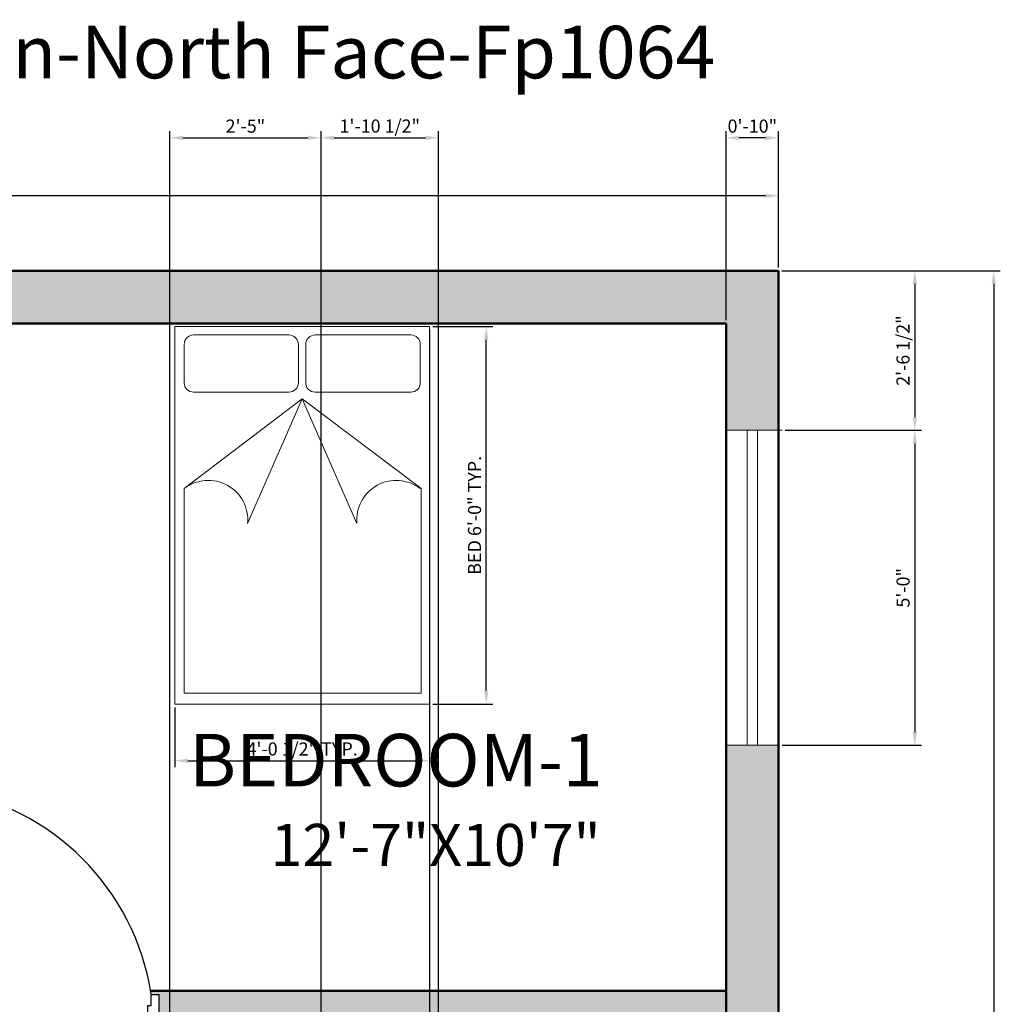
# Model space of a CAD drawing. Units: inches. Extents: x 3578 to 3951, y 1675 to 2189.
# Tile 4 of 4: x 3765 to 3951, y 2001 to 2189. Entities that reach past the tile are written whole.
import ezdxf

# ---------------------------------------------------------------- set-up
doc = ezdxf.new("R2010")
doc.units = ezdxf.units.IN
for name, color, linetype, lineweight in [('A-ANNO-DIMS', 2, 'Continuous', 18), ('A-ANNO-TEXT', 7, 'Continuous', 25), ('A-AREA-IDEN', 7, 'Continuous', 25), ('A-DOOR', 3, 'Continuous', 25), ('A-FURN', 8, 'Continuous', 18), ('A-GLAZ', 4, 'Continuous', 18), ('A-WALL', 7, 'Continuous', 50), ('A-WALL-PATT', 8, 'Continuous', 13)]:
    doc.layers.add(name, color=color, linetype=linetype, lineweight=lineweight)
doc.styles.get("Standard").update_dxf_attribs({"font": 'arial.ttf'})
doc.dimstyles.new('ISO-25', dxfattribs={"dimtxt": 2.5, "dimasz": 2.5, "dimexe": 1.25, "dimexo": 0.625, "dimtad": 1, "dimdec": 0, "dimlunit": 4, "dimtxsty": 'Standard', "dimcen": 2.5, "dimadec": 0, "dimazin": 0, "dimtfac": 1, "dimtdec": 0, "dimtmove": 0, "dimatfit": 3, "dimfxl": 1, "dimarcsym": 0})

# ---------------------------------------------------------------- blocks, each defined once
blk = doc.blocks.new('A$C36772BAF')
for p, q in [((0, 0), (0, 2)), ((0, 2), (1.35, 2)), ((1.35, 2), (1.35, 0)), ((0.6051, 1.9554), (0.1004, 1.9554)), ((1.2508, 1.9554), (0.7437, 1.9554)), ((0.0504, 1.9054), (0.0504, 1.7024)), ((0.6551, 1.9054), (0.6551, 1.7024)), ((0.6937, 1.9054), (0.6937, 1.7024)), ((1.3008, 1.7024), (1.3008, 1.9054)), ((0.1004, 1.6524), (0.6051, 1.6524)), ((0.7437, 1.6524), (1.2508, 1.6524)), ((0.6756, 1.6168), (0.0504, 1.1415)), ((0.386, 0.9573), (0.6756, 1.6168)), ((0.9651, 0.9573), (0.6756, 1.6168)), ((1.305, 1.1415), (0.6756, 1.6168)), ((0.0504, 1.1415), (0.0504, 0.0572)), ((1.305, 0.0572), (1.305, 1.1415)), ((0.0504, 0.0572), (1.305, 0.0572)), ((0, 0), (1.35, 0))]:
    blk.add_line(p, q)
for centre, radius, start, end in [((0.1004, 1.9054), 0.05, 90, 180), ((0.6051, 1.9054), 0.05, 0, 90), ((0.7437, 1.9054), 0.05, 90, 180), ((1.2508, 1.9054), 0.05, 0, 90), ((0.1004, 1.7024), 0.05, 180, 270), ((0.6051, 1.7024), 0.05, 270, 0), ((0.7437, 1.7024), 0.05, 180, 270), ((1.2508, 1.7024), 0.05, 270, 0), ((0.1778, 0.9758), 0.2091, 354.9358, 127.5591), ((1.1733, 0.9758), 0.2091, 52.4409, 185.0642)]:
    blk.add_arc(centre, radius, start, end)
blk = doc.blocks.new('A$C40E8097C')
for p, q in [((33.6, 192), (33.6, 1074.8)), ((72, 192), (72, 1068.3)), ((0, 192), (0, 0)), ((33.6, 192), (0, 192)), ((33.6, 144), (33.6, 192)), ((48, 144), (33.6, 144)), ((48, 48), (48, 144)), ((33.6, 0), (33.6, 48)), ((33.6, 48), (48, 48)), ((0, 0), (33.6, 0))]:
    blk.add_line(p, q)
blk.add_lwpolyline([(33.6, 192), (72, 192)])
blk.add_lwpolyline([(950, 192), (950, 0), (916.4, 0), (916.4, 48), (902, 48), (902, 144), (916.4, 144), (916.4, 192)], close=True)
blk.add_arc((-123.6, 34.8), 1051.8, 8.5964, 81.4036)
blk = doc.blocks.new('*D7')
at = {"layer": 'A-ANNO-DIMS', "color": 0, "lineweight": -2, "transparency": 16777216}
for p, q in [((3609.18, 2141.39), (3609.18, 2156.32)), ((3909.18, 2141.39), (3909.18, 2156.32)), ((3611.68, 2155.07), (3906.68, 2155.07))]:
    blk.add_line(p, q, dxfattribs=at)
at = {"layer": 'A-ANNO-DIMS', "color": 0, "transparency": 16777216}
for points in [[(3611.68, 2155.48), (3611.68, 2154.65), (3609.18, 2155.07)], [(3906.68, 2155.48), (3906.68, 2154.65), (3909.18, 2155.07)]]:
    blk.add_solid(points, dxfattribs=at)
at = {"layer": 'Defpoints', "color": 0, "transparency": 16777216}
for p in [(3909.18, 2155.07), (3609.18, 2140.77), (3909.18, 2140.77)]:
    blk.add_point(p, dxfattribs=at)
at = {"layer": 'A-ANNO-DIMS', "color": 0, "transparency": 16777216, "insert": (3759.18, 2156.97), "char_height": 2.5, "attachment_point": 5}
blk.add_mtext("25'", dxfattribs=at)
blk = doc.blocks.new('*D11')
at = {"layer": 'A-ANNO-DIMS', "color": 0, "lineweight": -2, "transparency": 16777216}
for p, q in [((3909.8, 2140.77), (3951.35, 2140.77)), ((3950.1, 2138.27), (3950.1, 1759.27)), ((3909.8, 1756.77), (3951.35, 1756.77))]:
    blk.add_line(p, q, dxfattribs=at)
at = {"layer": 'A-ANNO-DIMS', "color": 0, "transparency": 16777216}
for points in [[(3949.68, 2138.27), (3950.51, 2138.27), (3950.1, 2140.77)], [(3949.68, 1759.27), (3950.51, 1759.27), (3950.1, 1756.77)]]:
    blk.add_solid(points, dxfattribs=at)
at = {"layer": 'Defpoints', "color": 0, "transparency": 16777216}
for p in [(3909.18, 2140.77), (3909.18, 1756.77), (3950.1, 1756.77)]:
    blk.add_point(p, dxfattribs=at)
at = {"layer": 'A-ANNO-DIMS', "color": 0, "transparency": 16777216, "insert": (3948.19, 1948.77), "char_height": 2.5, "attachment_point": 5, "rotation": 90}
blk.add_mtext("32'", dxfattribs=at)
blk = doc.blocks.new('*D17')
at = {"layer": 'A-ANNO-DIMS', "color": 0, "lineweight": -2, "transparency": 16777216}
for p, q in [((3843.41, 2130.17), (3854.81, 2130.17)), ((3853.56, 2060.83), (3853.56, 2127.67)), ((3843.41, 2058.33), (3854.81, 2058.33))]:
    blk.add_line(p, q, dxfattribs=at)
at = {"layer": 'A-ANNO-DIMS', "color": 0, "transparency": 16777216}
for points in [[(3853.14, 2127.67), (3853.98, 2127.67), (3853.56, 2130.17)], [(3853.14, 2060.83), (3853.98, 2060.83), (3853.56, 2058.33)]]:
    blk.add_solid(points, dxfattribs=at)
at = {"layer": 'Defpoints', "color": 0, "transparency": 16777216}
for p in [(3842.79, 2130.17), (3853.56, 2130.17), (3842.79, 2058.33)]:
    blk.add_point(p, dxfattribs=at)
at = {"layer": 'A-ANNO-DIMS', "color": 0, "transparency": 16777216, "insert": (3851.66, 2094.25), "char_height": 2.5, "attachment_point": 5, "rotation": 90}
blk.add_mtext('BED 6\'-0" TYP.', dxfattribs=at)
blk = doc.blocks.new('*D18')
at = {"layer": 'A-ANNO-DIMS', "color": 0, "lineweight": -2, "transparency": 16777216}
for p, q in [((3794.3, 2057.71), (3794.3, 2046.31)), ((3842.79, 2057.71), (3842.79, 2046.31)), ((3796.8, 2047.56), (3840.29, 2047.56))]:
    blk.add_line(p, q, dxfattribs=at)
at = {"layer": 'A-ANNO-DIMS', "color": 0, "transparency": 16777216}
for points in [[(3796.8, 2047.97), (3796.8, 2047.14), (3794.3, 2047.56)], [(3840.29, 2047.97), (3840.29, 2047.14), (3842.79, 2047.56)]]:
    blk.add_solid(points, dxfattribs=at)
at = {"layer": 'Defpoints', "color": 0, "transparency": 16777216}
for p in [(3794.3, 2058.33), (3842.79, 2058.33), (3842.79, 2047.56)]:
    blk.add_point(p, dxfattribs=at)
at = {"layer": 'A-ANNO-DIMS', "color": 0, "transparency": 16777216, "insert": (3818.54, 2049.47), "char_height": 2.5, "attachment_point": 5}
blk.add_mtext('4\'-0 1/2" TYP.', dxfattribs=at)
blk = doc.blocks.new('*D31')
at = {"layer": 'A-ANNO-DIMS', "color": 0, "lineweight": -2, "transparency": 16777216}
for p, q in [((3909.8, 2140.77), (3936.33, 2140.77)), ((3935.08, 2138.27), (3935.08, 2112.92)), ((3910.45, 2110.42), (3936.33, 2110.42))]:
    blk.add_line(p, q, dxfattribs=at)
at = {"layer": 'A-ANNO-DIMS', "color": 0, "transparency": 16777216}
for points in [[(3934.66, 2138.27), (3935.5, 2138.27), (3935.08, 2140.77)], [(3934.66, 2112.92), (3935.5, 2112.92), (3935.08, 2110.42)]]:
    blk.add_solid(points, dxfattribs=at)
at = {"layer": 'Defpoints', "color": 0, "transparency": 16777216}
for p in [(3909.18, 2140.77), (3909.83, 2110.42), (3935.08, 2110.42)]:
    blk.add_point(p, dxfattribs=at)
at = {"layer": 'A-ANNO-DIMS', "color": 0, "transparency": 16777216, "insert": (3933.16, 2125.59), "char_height": 2.5, "attachment_point": 5, "rotation": 90}
blk.add_mtext('2\'-6 1/2"', dxfattribs=at)
blk = doc.blocks.new('*D32')
at = {"layer": 'A-ANNO-DIMS', "color": 0, "lineweight": -2, "transparency": 16777216}
for p, q in [((3910.45, 2110.42), (3936.33, 2110.42)), ((3935.08, 2107.92), (3935.08, 2053)), ((3909.88, 2050.5), (3936.33, 2050.5))]:
    blk.add_line(p, q, dxfattribs=at)
at = {"layer": 'A-ANNO-DIMS', "color": 0, "transparency": 16777216}
for points in [[(3934.66, 2107.92), (3935.5, 2107.92), (3935.08, 2110.42)], [(3934.66, 2053), (3935.5, 2053), (3935.08, 2050.5)]]:
    blk.add_solid(points, dxfattribs=at)
at = {"layer": 'Defpoints', "color": 0, "transparency": 16777216}
for p in [(3909.83, 2110.42), (3909.25, 2050.5), (3935.08, 2050.5)]:
    blk.add_point(p, dxfattribs=at)
at = {"layer": 'A-ANNO-DIMS', "color": 0, "transparency": 16777216, "insert": (3933.18, 2080.46), "char_height": 2.5, "attachment_point": 5, "rotation": 90}
blk.add_mtext('5\'-0"', dxfattribs=at)
blk = doc.blocks.new('*D43')
at = {"layer": 'A-ANNO-DIMS', "color": 0, "lineweight": -2, "transparency": 16777216}
for p, q in [((3822.14, 1757.39), (3822.14, 2167.33)), ((3824.64, 2166.08), (3841.99, 2166.08)), ((3844.49, 1757.39), (3844.49, 2167.33))]:
    blk.add_line(p, q, dxfattribs=at)
at = {"layer": 'A-ANNO-DIMS', "color": 0, "transparency": 16777216}
for points in [[(3824.64, 2166.49), (3824.64, 2165.66), (3822.14, 2166.08)], [(3841.99, 2166.49), (3841.99, 2165.66), (3844.49, 2166.08)]]:
    blk.add_solid(points, dxfattribs=at)
at = {"layer": 'Defpoints', "color": 0, "transparency": 16777216}
for p in [(3844.49, 2166.08), (3822.14, 1756.77), (3844.49, 1756.77)]:
    blk.add_point(p, dxfattribs=at)
at = {"layer": 'A-ANNO-DIMS', "color": 0, "transparency": 16777216, "insert": (3833.31, 2167.99), "char_height": 2.5, "attachment_point": 5}
blk.add_mtext('1\'-10 1/2"', dxfattribs=at)
blk = doc.blocks.new('*D45')
at = {"layer": 'A-ANNO-DIMS', "color": 0, "lineweight": -2, "transparency": 16777216}
for p, q in [((3899.18, 2131.39), (3899.18, 2167.33)), ((3906.68, 2166.08), (3901.68, 2166.08)), ((3909.18, 2141.39), (3909.18, 2167.33))]:
    blk.add_line(p, q, dxfattribs=at)
at = {"layer": 'A-ANNO-DIMS', "color": 0, "transparency": 16777216}
for points in [[(3901.68, 2166.49), (3901.68, 2165.66), (3899.18, 2166.08)], [(3906.68, 2166.49), (3906.68, 2165.66), (3909.18, 2166.08)]]:
    blk.add_solid(points, dxfattribs=at)
at = {"layer": 'Defpoints', "color": 0, "transparency": 16777216}
for p in [(3899.18, 2166.08), (3909.18, 2140.77), (3899.18, 2130.77)]:
    blk.add_point(p, dxfattribs=at)
at = {"layer": 'A-ANNO-DIMS', "color": 0, "transparency": 16777216, "insert": (3904.18, 2167.98), "char_height": 2.5, "attachment_point": 5}
blk.add_mtext('0\'-10"', dxfattribs=at)
blk = doc.blocks.new('*D56')
at = {"layer": 'A-ANNO-DIMS', "color": 0, "lineweight": -2, "transparency": 16777216}
for p, q in [((3899.18, 2130.14), (3899.18, 1696.88)), ((3842.79, 2129.55), (3842.79, 1696.88)), ((3896.68, 1698.13), (3845.29, 1698.13))]:
    blk.add_line(p, q, dxfattribs=at)
at = {"layer": 'A-ANNO-DIMS', "color": 0, "transparency": 16777216}
for points in [[(3845.29, 1698.55), (3845.29, 1697.71), (3842.79, 1698.13)], [(3896.68, 1698.55), (3896.68, 1697.71), (3899.18, 1698.13)]]:
    blk.add_solid(points, dxfattribs=at)
at = {"layer": 'Defpoints', "color": 0, "transparency": 16777216}
for p in [(3842.79, 2130.17), (3899.18, 2130.77), (3842.79, 1698.13)]:
    blk.add_point(p, dxfattribs=at)
at = {"layer": 'A-ANNO-DIMS', "color": 0, "transparency": 16777216, "insert": (3870.98, 1700.05), "char_height": 2.5, "attachment_point": 5}
blk.add_mtext('4\'-8 1/2"', dxfattribs=at)
blk = doc.blocks.new('*D59')
at = {"layer": 'A-ANNO-DIMS', "color": 0, "lineweight": -2, "transparency": 16777216}
for p, q in [((3793.35, 1768.19), (3793.35, 2167.33)), ((3795.85, 2166.08), (3819.64, 2166.08)), ((3822.14, 1767.4), (3822.14, 2167.33))]:
    blk.add_line(p, q, dxfattribs=at)
at = {"layer": 'A-ANNO-DIMS', "color": 0, "transparency": 16777216}
for points in [[(3795.85, 2166.49), (3795.85, 2165.66), (3793.35, 2166.08)], [(3819.64, 2166.49), (3819.64, 2165.66), (3822.14, 2166.08)]]:
    blk.add_solid(points, dxfattribs=at)
at = {"layer": 'Defpoints', "color": 0, "transparency": 16777216}
for p in [(3822.14, 2166.08), (3793.35, 1767.57), (3822.14, 1766.77)]:
    blk.add_point(p, dxfattribs=at)
at = {"layer": 'A-ANNO-DIMS', "color": 0, "transparency": 16777216, "insert": (3807.75, 2167.98), "char_height": 2.5, "attachment_point": 5}
blk.add_mtext('2\'-5"', dxfattribs=at)

msp = doc.modelspace()

# ---------------------------------------------------------------- hatches: boundary and pattern name
at = {"layer": 'A-WALL-PATT'}
h = msp.add_hatch(color=256, dxfattribs=at)
h.dxf.hatch_style = 1
h.paths.add_polyline_path([(3619.18, 1950.71), (3609.18, 1950.71), (3609.18, 1756.77), (3648.78, 1756.77), (3648.78, 1766.77), (3619.18, 1766.77)])
h.paths.add_polyline_path([(3619.18, 2068.71), (3609.18, 2068.71), (3609.18, 1975.57), (3619.18, 1975.57), (3619.18, 1998.77)])
h.paths.add_polyline_path([(3619.18, 2130.77), (3647.07, 2130.77), (3647.07, 2140.77), (3609.18, 2140.77), (3609.18, 2104.48), (3619.18, 2104.48)])
h.paths.add_polyline_path([(3909.18, 2140.77), (3713.13, 2140.77), (3713.13, 2130.77), (3899.18, 2130.77), (3899.18, 2110.42), (3909.18, 2110.42)])
h.paths.add_polyline_path([(3909.18, 2050.5), (3899.18, 2050.5), (3899.18, 1980.99), (3909.18, 1980.99)])
h.paths.add_polyline_path([(3909.18, 1881.86), (3899.18, 1881.86), (3899.18, 1941.89), (3890.7, 1942.45), (3889.21, 1942.68, -0.02009), (3881.89, 1944.66, -0.072677), (3876.18, 1946.94, -0.17277), (3874.16, 1950.75, -0.17277), (3875.79, 1954.64, -0.055418), (3880.27, 1956.72, -0.024581), (3889.21, 1959.22), (3890.7, 1959.45), (3899.18, 1960.01), (3899.18, 1952.98), (3909.18, 1952.98)])
h.paths.add_polyline_path([(3891.56, 1958.83, 0.100666), (3890.28, 1958.86, 0.024932), (3881.25, 1956.42, 0.064314), (3876.22, 1954.24, 0.17277), (3874.74, 1950.82, 0.17277), (3876.47, 1947.45, 0.072922), (3882.04, 1945.22, 0.022708), (3890.28, 1943.04, 0.100666), (3891.56, 1943.07, 0.125847)], flags=16)
h.paths.add_polyline_path([(3898.92, 1942.47, 0.324885), (3899.15, 1942.79), (3899.15, 1959.11, 0.551642), (3898.67, 1959.41), (3899.15, 1959.45), (3899.15, 1942.45)], flags=16)
h.paths.add_polyline_path([(3890.7, 1948.47, -1), (3891.63, 1948.47, -1)], flags=0)
h.paths.add_polyline_path([(3884.71, 1945.94, -0.104302), (3877.06, 1948.46, -0.17277), (3875.9, 1950.94, -0.17277), (3877.06, 1953.43, -0.104302), (3884.71, 1955.94, -0.414214), (3889.71, 1950.94, -0.414214)], flags=0)
h.paths.add_polyline_path([(3887.07, 1948.79), (3885.02, 1950.11, -0.031181), (3884.52, 1950.35, -0.229141), (3884.09, 1950.94, -0.229141), (3884.52, 1951.54, -0.109107), (3886.35, 1952.09, -0.199237), (3886.5, 1952.04, -0.461153), (3886.5, 1949.84), (3887.38, 1949.28)], flags=0)
h.paths.add_polyline_path([(3890.7, 1953.43, -1), (3891.63, 1953.43, -1)], flags=0)
h.paths.add_polyline_path([(3909.18, 1843.84), (3899.18, 1843.84), (3899.18, 1766.77), (3844.49, 1766.77), (3844.49, 1756.77), (3909.18, 1756.77)])
h = msp.add_hatch(color=256, dxfattribs=at)
h.dxf.hatch_style = 1
h.paths.add_polyline_path([(3899.18, 2003.77), (3789.71, 2003.77, -0.003692), (3789.81, 2003.09), (3791.29, 2003.09), (3791.29, 1998.77), (3899.18, 1998.77)])
h.paths.add_polyline_path([(3748.18, 2130.77), (3743.18, 2130.77), (3743.18, 2003.77), (3748.18, 2003.77)])
h.paths.add_polyline_path([(3899.18, 1920.77), (3864.53, 1920.77), (3864.53, 1915.77), (3899.18, 1915.77)], flags=0)
h.paths.add_polyline_path([(3748.18, 1872.53), (3743.18, 1872.53), (3743.18, 1766.77), (3748.18, 1766.77)], flags=0)
h.paths.add_polyline_path([(3807.15, 1834.35), (3847.1, 1834.35), (3847.1, 1854.95), (3807.15, 1854.95)], flags=8)
h.paths.add_polyline_path([(3791.36, 1816.7), (3859.75, 1816.7), (3859.75, 1833.18), (3791.36, 1833.18)], flags=8)
h.paths.add_polyline_path([(3771.09, 1986.79), (3779.29, 1986.79), (3779.29, 1991.94), (3771.09, 1991.94)], flags=8)
h.paths.add_polyline_path([(3782.02, 1935.64), (3790.22, 1935.64), (3790.22, 1940.79), (3782.02, 1940.79)], flags=8)

# ---------------------------------------------------------------- linework, layer by layer
at = {"layer": 'A-GLAZ'}
for p, q in [((3909.83, 2110.42), (3899.18, 2110.42)), ((3903.18, 2110.42), (3903.18, 2050.5)), ((3905.18, 2110.42), (3905.18, 2050.5)), ((3899.18, 2050.5), (3909.25, 2050.5))]:
    msp.add_line(p, q, dxfattribs=at)
at = {"layer": 'A-WALL'}
for p, q in [((3609.18, 2140.77), (3909.18, 2140.77)), ((3909.18, 2140.77), (3909.18, 1756.77)), ((3619.18, 2130.77), (3899.18, 2130.77)), ((3899.18, 2130.77), (3899.18, 1766.77)), ((3789.71, 2003.77), (3899.18, 2003.77))]:
    msp.add_line(p, q, dxfattribs=at)

# ---------------------------------------------------------------- block references
at = {"layer": 'A-DOOR', "xscale": 0.044006868052547, "yscale": 0.044006868052547, "zscale": 0.044006868052547}
msp.add_blockref('A$C40E8097C', (3749.49, 1994.64), dxfattribs=at)
at = {"layer": 'A-FURN', "xscale": 35.91900852829305, "yscale": 35.91900852829305, "zscale": 35.91900852829305}
msp.add_blockref('A$C36772BAF', (3794.3, 2058.33), dxfattribs=at)

# ---------------------------------------------------------------- texts
at = {"layer": 'A-ANNO-TEXT', "insert": (3617.08, 2187.39), "char_height": 10, "attachment_point": 1}
msp.add_mtext('25X32(800ft) House Plan-North Face-Fp1064', dxfattribs=at)
at = {"layer": 'A-AREA-IDEN', "attachment_point": 1}
for s, insert, char_height in [('BEDROOM-1', (3797.02, 2052.66), 10), ('12\'-7"X10\'7"', (3812.54, 2035.54), 8)]:
    msp.add_mtext(s, dxfattribs=dict(at, insert=insert, char_height=char_height))

# ---------------------------------------------------------------- dimensions: what is measured, and where the dimension line sits
at = {"layer": 'A-ANNO-DIMS'}
for base, p1, p2, override, picture, middle in [((3844.4921, 2166.0767), (3822.1369, 1756.7652), (3844.4921, 1756.7652), {"dimdec": 1, "dimlfac": 1, "dimrnd": 0, "dimzin": 1, "dimdsep": 46, "dimlunit": 4, "dimfrac": 2}, '*D43', (3833.3145, 2167.9944)), ((3822.14, 2166.08), (3793.35, 1767.57), (3822.14, 1766.77), {"dimdec": 1, "dimlfac": 1, "dimrnd": 0, "dimzin": 1, "dimdsep": 46, "dimlunit": 4, "dimfrac": 2}, '*D59', (3807.75, 2167.98)), ((3899.18, 2166.08), (3909.18, 2140.77), (3899.18, 2130.77), {"dimdec": 1, "dimlfac": 1, "dimrnd": 0, "dimzin": 1, "dimdsep": 46, "dimlunit": 4, "dimfrac": 2}, '*D45', (3904.18, 2167.98)), ((3909.18, 2155.07), (3609.18, 2140.77), (3909.18, 2140.77), {"dimclrd": 0, "dimclre": 0, "dimclrt": 0}, '*D7', (3759.18, 2156.97)), ((3842.79, 1698.13), (3899.18, 2130.77), (3842.79, 2130.17), {"dimdec": 1, "dimlfac": 1, "dimrnd": 0, "dimzin": 1, "dimdsep": 46, "dimlunit": 4, "dimfrac": 2}, '*D56', (3870.98, 1700.05))]:
    dim = msp.add_linear_dim(base=base, p1=p1, p2=p2, dimstyle='ISO-25', override=override, dxfattribs=at)
    dim.commit()
    dim.dimension.update_dxf_attribs({"geometry": picture, "text_midpoint": middle})
for base, p1, p2, override, picture, middle in [((3950.1, 1756.77), (3909.18, 2140.77), (3909.18, 1756.77), {"dimclrd": 0, "dimclre": 0, "dimclrt": 0}, '*D11', (3948.19, 1948.77)), ((3935.0794, 2110.4189), (3909.1796, 2140.7652), (3909.8294, 2110.4189), {"dimdec": 1, "dimlfac": 1, "dimrnd": 0, "dimzin": 1, "dimdsep": 46, "dimlunit": 4, "dimfrac": 2}, '*D31', (3933.1618, 2125.5921)), ((3935.08, 2050.5), (3909.83, 2110.42), (3909.25, 2050.5), {"dimdec": 1, "dimlfac": 1, "dimrnd": 0, "dimzin": 1, "dimdsep": 46, "dimlunit": 4, "dimfrac": 2}, '*D32', (3933.18, 2080.46))]:
    dim = msp.add_linear_dim(base=base, p1=p1, p2=p2, angle=90, dimstyle='ISO-25', override=override, dxfattribs=at)
    dim.commit()
    dim.dimension.update_dxf_attribs({"geometry": picture, "text_midpoint": middle})
dim = msp.add_linear_dim(base=(3853.56, 2130.17), p1=(3842.79, 2058.33), p2=(3842.79, 2130.17), angle=90, text='BED <> TYP.', dimstyle='ISO-25', override={"dimdec": 1, "dimlfac": 1, "dimrnd": 0, "dimzin": 1, "dimdsep": 46, "dimlunit": 4, "dimfrac": 2}, dxfattribs=at)
dim.commit()
dim.dimension.update_dxf_attribs({"geometry": '*D17', "text_midpoint": (3851.66, 2094.25)})
dim = msp.add_linear_dim(base=(3842.79, 2047.56), p1=(3794.3, 2058.33), p2=(3842.79, 2058.33), text='<> TYP.', dimstyle='ISO-25', override={"dimdec": 1, "dimlfac": 1, "dimrnd": 0, "dimzin": 1, "dimdsep": 46, "dimlunit": 4, "dimfrac": 2}, dxfattribs=at)
dim.commit()
dim.dimension.update_dxf_attribs({"geometry": '*D18', "text_midpoint": (3818.54, 2049.47)})

doc.saveas('drawing.dxf')
